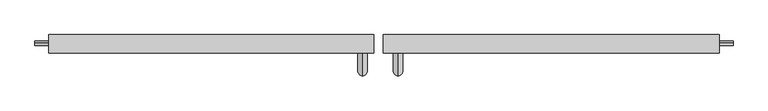
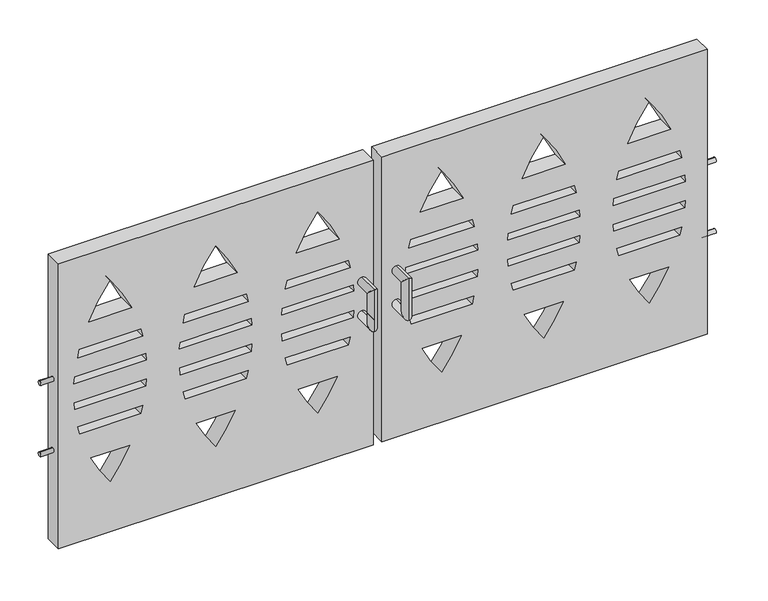
"""IFC4 building model written with IfcOpenShell, lengths in millimetres: proxy geometry."""

from ifc_helpers import new_model, si_unit, point, frame, frame_2d, origin, place, context, project, spatial, polyline, circle_curve, ellipse_curve, trimmed, segment, composite_curve, outline, extrude, source, transform, mapped, element, save
from ifc_brep_helpers import plane_surface, cylinder_surface, advanced_brep


def generic_models_afecbd1f(model_context):
    return source(origin(), model_context, "Body", "SolidModel", [
        extrude(outline(polyline([(0.0, 268.7654616), (1727.2, 268.7654616), (1727.2, -1534.6345384), (0.0, -1534.6345384), (0.0, 268.7654616)]), holes=[composite_curve([segment(trimmed(circle_curve(frame_2d((913.3858921, 735.2120442)), 991.7835907), [point((1315.7032602, -171.3062546))], [point((1522.0610264, -47.8264425))], True, "CARTESIAN"), True, "CONTINUOUS"), segment(trimmed(circle_curve(frame_2d((913.3858921, -830.8649293)), 991.7835907), [point((1522.0610264, -47.8264425))], [point((1315.7032602, 75.6533695))], True, "CARTESIAN"), True, "CONTINUOUS"), segment(polyline([(1315.7032602, 75.6533695), (1315.7032602, -171.3062546)]), True, "CONTINUOUS")], self_intersect=False), composite_curve([segment(trimmed(circle_curve(frame_2d((913.3858921, -830.8649293)), 991.7835907), [point((1167.7706197, 127.7398387))], [point((1120.5108318, 139.0494742))], True, "CARTESIAN"), True, "CONTINUOUS"), segment(polyline([(1120.5108318, 139.0494742), (1120.5108318, -234.7023593)]), True, "CONTINUOUS"), segment(trimmed(circle_curve(frame_2d((913.3858921, 735.2120442)), 991.7835907), [point((1120.5108318, -234.7023593))], [point((1167.7706197, -223.3927238))], True, "CARTESIAN"), True, "CONTINUOUS"), segment(polyline([(1167.7706197, -223.3927238), (1167.7706197, 127.7398387)]), True, "CONTINUOUS")], self_intersect=False), composite_curve([segment(trimmed(circle_curve(frame_2d((913.3858921, -830.8649293)), 991.7835907), [point((1008.9376367, 156.3050434))], [point((969.7809206, 159.3139897))], True, "CARTESIAN"), True, "CONTINUOUS"), segment(polyline([(969.7809206, 159.3139897), (969.7809206, -254.9668748)]), True, "CONTINUOUS"), segment(trimmed(circle_curve(frame_2d((913.3858921, 735.2120442)), 991.7835907), [point((969.7809206, -254.9668748))], [point((1008.9376367, -251.9579284))], True, "CARTESIAN"), True, "CONTINUOUS"), segment(polyline([(1008.9376367, -251.9579284), (1008.9376367, 156.3050434)]), True, "CONTINUOUS")], self_intersect=False), composite_curve([segment(trimmed(circle_curve(frame_2d((913.3858921, -830.8649293)), 991.7835907), [point((853.4628105, 159.1067446))], [point((811.4921317, 155.6706009))], True, "CARTESIAN"), True, "CONTINUOUS"), segment(polyline([(811.4921317, 155.6706009), (811.4921317, -251.323486)]), True, "CONTINUOUS"), segment(trimmed(circle_curve(frame_2d((913.3858921, 735.2120442)), 991.7835907), [point((811.4921317, -251.323486))], [point((853.4628105, -254.7596297))], True, "CARTESIAN"), True, "CONTINUOUS"), segment(polyline([(853.4628105, -254.7596297), (853.4628105, 159.1067446)]), True, "CONTINUOUS")], self_intersect=False), composite_curve([segment(trimmed(circle_curve(frame_2d((913.3858921, -830.8649293)), 991.7835907), [point((700.6764218, 137.8400681))], [point((655.683383, 126.8532483))], True, "CARTESIAN"), True, "CONTINUOUS"), segment(polyline([(655.683383, 126.8532483), (655.683383, -222.5061333)]), True, "CONTINUOUS"), segment(trimmed(circle_curve(frame_2d((913.3858921, 735.2120442)), 991.7835907), [point((655.683383, -222.5061333))], [point((700.6764218, -233.4929532))], True, "CARTESIAN"), True, "CONTINUOUS"), segment(polyline([(700.6764218, -233.4929532), (700.6764218, 137.8400681)]), True, "CONTINUOUS")], self_intersect=False), composite_curve([segment(trimmed(circle_curve(frame_2d((913.3858921, -830.8649293)), 991.7835907), [point((485.5755246, 63.9048625))], [point((304.7107578, -47.8264425))], True, "CARTESIAN"), True, "CONTINUOUS"), segment(trimmed(circle_curve(frame_2d((913.3858921, 735.2120442)), 991.7835907), [point((304.7107578, -47.8264425))], [point((485.5755246, -159.5577476))], True, "CARTESIAN"), True, "CONTINUOUS"), segment(polyline([(485.5755246, -159.5577476), (485.5755246, 63.9048625)]), True, "CONTINUOUS")], self_intersect=False), composite_curve([segment(polyline([(1315.7032602, -510.0774949), (1315.7032602, -757.0371191)]), True, "CONTINUOUS"), segment(trimmed(circle_curve(frame_2d((913.3858921, 149.4811798)), 991.7835907), [point((1315.7032602, -757.0371191))], [point((1522.0610264, -633.557307))], True, "CARTESIAN"), True, "CONTINUOUS"), segment(trimmed(circle_curve(frame_2d((913.3858921, -1416.5957937)), 991.7835907), [point((1522.0610264, -633.557307))], [point((1315.7032602, -510.0774949))], True, "CARTESIAN"), True, "CONTINUOUS")], self_intersect=False), composite_curve([segment(polyline([(1167.7706197, -809.1235882), (1167.7706197, -457.9910257)]), True, "CONTINUOUS"), segment(trimmed(circle_curve(frame_2d((913.3858921, -1416.5957937)), 991.7835907), [point((1167.7706197, -457.9910257))], [point((1120.5108318, -446.6813902))], True, "CARTESIAN"), True, "CONTINUOUS"), segment(polyline([(1120.5108318, -446.6813902), (1120.5108318, -820.4332237)]), True, "CONTINUOUS"), segment(trimmed(circle_curve(frame_2d((913.3858921, 149.4811798)), 991.7835907), [point((1120.5108318, -820.4332237))], [point((1167.7706197, -809.1235882))], True, "CARTESIAN"), True, "CONTINUOUS")], self_intersect=False), composite_curve([segment(polyline([(1008.9376367, -837.6887929), (1008.9376367, -429.4258211)]), True, "CONTINUOUS"), segment(trimmed(circle_curve(frame_2d((913.3858921, -1416.5957937)), 991.7835907), [point((1008.9376367, -429.4258211))], [point((969.7809206, -426.4168748))], True, "CARTESIAN"), True, "CONTINUOUS"), segment(polyline([(969.7809206, -426.4168748), (969.7809206, -840.6977392)]), True, "CONTINUOUS"), segment(trimmed(circle_curve(frame_2d((913.3858921, 149.4811798)), 991.7835907), [point((969.7809206, -840.6977392))], [point((1008.9376367, -837.6887929))], True, "CARTESIAN"), True, "CONTINUOUS")], self_intersect=False), composite_curve([segment(polyline([(853.4628105, -840.4904941), (853.4628105, -426.6241198)]), True, "CONTINUOUS"), segment(trimmed(circle_curve(frame_2d((913.3858921, -1416.5957937)), 991.7835907), [point((853.4628105, -426.6241198))], [point((811.4921317, -430.0602635))], True, "CARTESIAN"), True, "CONTINUOUS"), segment(polyline([(811.4921317, -430.0602635), (811.4921317, -837.0543504)]), True, "CONTINUOUS"), segment(trimmed(circle_curve(frame_2d((913.3858921, 149.4811798)), 991.7835907), [point((811.4921317, -837.0543504))], [point((853.4628105, -840.4904941))], True, "CARTESIAN"), True, "CONTINUOUS")], self_intersect=False), composite_curve([segment(polyline([(700.6764218, -819.2238176), (700.6764218, -447.8907963)]), True, "CONTINUOUS"), segment(trimmed(circle_curve(frame_2d((913.3858921, -1416.5957937)), 991.7835907), [point((700.6764218, -447.8907963))], [point((655.683383, -458.8776162))], True, "CARTESIAN"), True, "CONTINUOUS"), segment(polyline([(655.683383, -458.8776162), (655.683383, -808.2369978)]), True, "CONTINUOUS"), segment(trimmed(circle_curve(frame_2d((913.3858921, 149.4811798)), 991.7835907), [point((655.683383, -808.2369978))], [point((700.6764218, -819.2238176))], True, "CARTESIAN"), True, "CONTINUOUS")], self_intersect=False), composite_curve([segment(polyline([(485.5755246, -745.288612), (485.5755246, -521.8260019)]), True, "CONTINUOUS"), segment(trimmed(circle_curve(frame_2d((913.3858921, -1416.5957937)), 991.7835907), [point((485.5755246, -521.8260019))], [point((304.7107578, -633.557307))], True, "CARTESIAN"), True, "CONTINUOUS"), segment(trimmed(circle_curve(frame_2d((913.3858921, 149.4811798)), 991.7835907), [point((304.7107578, -633.557307))], [point((485.5755246, -745.288612))], True, "CARTESIAN"), True, "CONTINUOUS")], self_intersect=False), composite_curve([segment(trimmed(circle_curve(frame_2d((913.3858921, -455.2996847)), 991.7835907), [point((1315.7032602, -1361.8179835))], [point((1522.0610264, -1238.3381714))], True, "CARTESIAN"), True, "CONTINUOUS"), segment(trimmed(circle_curve(frame_2d((913.3858921, -2021.3766581)), 991.7835907), [point((1522.0610264, -1238.3381714))], [point((1315.7032602, -1114.8583593))], True, "CARTESIAN"), True, "CONTINUOUS"), segment(polyline([(1315.7032602, -1114.8583593), (1315.7032602, -1361.8179835)]), True, "CONTINUOUS")], self_intersect=False), composite_curve([segment(trimmed(circle_curve(frame_2d((913.3858921, -2021.3766581)), 991.7835907), [point((1167.7706197, -1062.7718902))], [point((1120.5108318, -1051.4622546))], True, "CARTESIAN"), True, "CONTINUOUS"), segment(polyline([(1120.5108318, -1051.4622546), (1120.5108318, -1425.2140882)]), True, "CONTINUOUS"), segment(trimmed(circle_curve(frame_2d((913.3858921, -455.2996847)), 991.7835907), [point((1120.5108318, -1425.2140882))], [point((1167.7706197, -1413.9044526))], True, "CARTESIAN"), True, "CONTINUOUS"), segment(polyline([(1167.7706197, -1413.9044526), (1167.7706197, -1062.7718902)]), True, "CONTINUOUS")], self_intersect=False), composite_curve([segment(trimmed(circle_curve(frame_2d((913.3858921, -2021.3766581)), 991.7835907), [point((1008.9376367, -1034.2066855))], [point((969.7809206, -1031.1977392))], True, "CARTESIAN"), True, "CONTINUOUS"), segment(polyline([(969.7809206, -1031.1977392), (969.7809206, -1445.4786036)]), True, "CONTINUOUS"), segment(trimmed(circle_curve(frame_2d((913.3858921, -455.2996847)), 991.7835907), [point((969.7809206, -1445.4786036))], [point((1008.9376367, -1442.4696573))], True, "CARTESIAN"), True, "CONTINUOUS"), segment(polyline([(1008.9376367, -1442.4696573), (1008.9376367, -1034.2066855)]), True, "CONTINUOUS")], self_intersect=False), composite_curve([segment(trimmed(circle_curve(frame_2d((913.3858921, -2021.3766581)), 991.7835907), [point((853.4628105, -1031.4049843))], [point((811.4921317, -1034.8411279))], True, "CARTESIAN"), True, "CONTINUOUS"), segment(polyline([(811.4921317, -1034.8411279), (811.4921317, -1441.8352149)]), True, "CONTINUOUS"), segment(trimmed(circle_curve(frame_2d((913.3858921, -455.2996847)), 991.7835907), [point((811.4921317, -1441.8352149))], [point((853.4628105, -1445.2713585))], True, "CARTESIAN"), True, "CONTINUOUS"), segment(polyline([(853.4628105, -1445.2713585), (853.4628105, -1031.4049843)]), True, "CONTINUOUS")], self_intersect=False), composite_curve([segment(trimmed(circle_curve(frame_2d((913.3858921, -2021.3766581)), 991.7835907), [point((700.6764218, -1052.6716607))], [point((655.683383, -1063.6584806))], True, "CARTESIAN"), True, "CONTINUOUS"), segment(polyline([(655.683383, -1063.6584806), (655.683383, -1413.0178622)]), True, "CONTINUOUS"), segment(trimmed(circle_curve(frame_2d((913.3858921, -455.2996847)), 991.7835907), [point((655.683383, -1413.0178622))], [point((700.6764218, -1424.0046821))], True, "CARTESIAN"), True, "CONTINUOUS"), segment(polyline([(700.6764218, -1424.0046821), (700.6764218, -1052.6716607)]), True, "CONTINUOUS")], self_intersect=False), composite_curve([segment(trimmed(circle_curve(frame_2d((913.3858921, -2021.3766581)), 991.7835907), [point((485.5755246, -1126.6068664))], [point((304.7107578, -1238.3381714))], True, "CARTESIAN"), True, "CONTINUOUS"), segment(trimmed(circle_curve(frame_2d((913.3858921, -455.2996847)), 991.7835907), [point((304.7107578, -1238.3381714))], [point((485.5755246, -1350.0694764))], True, "CARTESIAN"), True, "CONTINUOUS"), segment(polyline([(485.5755246, -1350.0694764), (485.5755246, -1126.6068664)]), True, "CONTINUOUS")], self_intersect=False)]), frame((0.0, -101.6, 0.0), z_axis=(0.0, 1.0, 0.0), x_axis=(0.0, 0.0, 1.0)), (0.0, 0.0, 1.0), 101.6),
        extrude(outline(polyline([(1727.2, 2183.266195), (1727.2, 319.5654616), (0.0, 319.5654616), (0.0, 2183.266195), (1727.2, 2183.266195)]), holes=[composite_curve([segment(polyline([(1315.7032602, 785.0371778), (1315.7032602, 538.0775536)]), True, "CONTINUOUS"), segment(trimmed(circle_curve(frame_2d((913.3858921, 1444.5958525)), 991.7835907), [point((1315.7032602, 538.0775536))], [point((1522.0610264, 661.5573657))], True, "CARTESIAN"), True, "CONTINUOUS"), segment(trimmed(circle_curve(frame_2d((913.3858921, -121.481121)), 991.7835907), [point((1522.0610264, 661.5573657))], [point((1315.7032602, 785.0371778))], True, "CARTESIAN"), True, "CONTINUOUS")], self_intersect=False), composite_curve([segment(polyline([(1167.7706197, 485.9910845), (1167.7706197, 837.1236469)]), True, "CONTINUOUS"), segment(trimmed(circle_curve(frame_2d((913.3858921, -121.481121)), 991.7835907), [point((1167.7706197, 837.1236469))], [point((1120.5108318, 848.4332825))], True, "CARTESIAN"), True, "CONTINUOUS"), segment(polyline([(1120.5108318, 848.4332825), (1120.5108318, 474.681449)]), True, "CONTINUOUS"), segment(trimmed(circle_curve(frame_2d((913.3858921, 1444.5958525)), 991.7835907), [point((1120.5108318, 474.681449))], [point((1167.7706197, 485.9910845))], True, "CARTESIAN"), True, "CONTINUOUS")], self_intersect=False), composite_curve([segment(polyline([(1008.9376367, 457.4258798), (1008.9376367, 865.6888516)]), True, "CONTINUOUS"), segment(trimmed(circle_curve(frame_2d((913.3858921, -121.481121)), 991.7835907), [point((1008.9376367, 865.6888516))], [point((969.7809206, 868.6977979))], True, "CARTESIAN"), True, "CONTINUOUS"), segment(polyline([(969.7809206, 868.6977979), (969.7809206, 454.4169335)]), True, "CONTINUOUS"), segment(trimmed(circle_curve(frame_2d((913.3858921, 1444.5958525)), 991.7835907), [point((969.7809206, 454.4169335))], [point((1008.9376367, 457.4258798))], True, "CARTESIAN"), True, "CONTINUOUS")], self_intersect=False), composite_curve([segment(polyline([(853.4628105, 454.6241786), (853.4628105, 868.4905529)]), True, "CONTINUOUS"), segment(trimmed(circle_curve(frame_2d((913.3858921, -121.481121)), 991.7835907), [point((853.4628105, 868.4905529))], [point((811.4921317, 865.0544092))], True, "CARTESIAN"), True, "CONTINUOUS"), segment(polyline([(811.4921317, 865.0544092), (811.4921317, 458.0603222)]), True, "CONTINUOUS"), segment(trimmed(circle_curve(frame_2d((913.3858921, 1444.5958525)), 991.7835907), [point((811.4921317, 458.0603222))], [point((853.4628105, 454.6241786))], True, "CARTESIAN"), True, "CONTINUOUS")], self_intersect=False), composite_curve([segment(polyline([(700.6764218, 475.890855), (700.6764218, 847.2238764)]), True, "CONTINUOUS"), segment(trimmed(circle_curve(frame_2d((913.3858921, -121.481121)), 991.7835907), [point((700.6764218, 847.2238764))], [point((655.683383, 836.2370565))], True, "CARTESIAN"), True, "CONTINUOUS"), segment(polyline([(655.683383, 836.2370565), (655.683383, 486.8776749)]), True, "CONTINUOUS"), segment(trimmed(circle_curve(frame_2d((913.3858921, 1444.5958525)), 991.7835907), [point((655.683383, 486.8776749))], [point((700.6764218, 475.890855))], True, "CARTESIAN"), True, "CONTINUOUS")], self_intersect=False), composite_curve([segment(polyline([(485.5755246, 549.8260607), (485.5755246, 773.2886707)]), True, "CONTINUOUS"), segment(trimmed(circle_curve(frame_2d((913.3858921, -121.481121)), 991.7835907), [point((485.5755246, 773.2886707))], [point((304.7107578, 661.5573657))], True, "CARTESIAN"), True, "CONTINUOUS"), segment(trimmed(circle_curve(frame_2d((913.3858921, 1444.5958525)), 991.7835907), [point((304.7107578, 661.5573657))], [point((485.5755246, 549.8260607))], True, "CARTESIAN"), True, "CONTINUOUS")], self_intersect=False), composite_curve([segment(trimmed(circle_curve(frame_2d((913.3858921, 2030.3267169)), 991.7835907), [point((1315.7032602, 1123.8084181))], [point((1522.0610264, 1247.2882301))], True, "CARTESIAN"), True, "CONTINUOUS"), segment(trimmed(circle_curve(frame_2d((913.3858921, 464.2497434)), 991.7835907), [point((1522.0610264, 1247.2882301))], [point((1315.7032602, 1370.7680422))], True, "CARTESIAN"), True, "CONTINUOUS"), segment(polyline([(1315.7032602, 1370.7680422), (1315.7032602, 1123.8084181)]), True, "CONTINUOUS")], self_intersect=False), composite_curve([segment(trimmed(circle_curve(frame_2d((913.3858921, 464.2497434)), 991.7835907), [point((1167.7706197, 1422.8545114))], [point((1120.5108318, 1434.1641469))], True, "CARTESIAN"), True, "CONTINUOUS"), segment(polyline([(1120.5108318, 1434.1641469), (1120.5108318, 1060.4123134)]), True, "CONTINUOUS"), segment(trimmed(circle_curve(frame_2d((913.3858921, 2030.3267169)), 991.7835907), [point((1120.5108318, 1060.4123134))], [point((1167.7706197, 1071.7219489))], True, "CARTESIAN"), True, "CONTINUOUS"), segment(polyline([(1167.7706197, 1071.7219489), (1167.7706197, 1422.8545114)]), True, "CONTINUOUS")], self_intersect=False), composite_curve([segment(trimmed(circle_curve(frame_2d((913.3858921, 464.2497434)), 991.7835907), [point((1008.9376367, 1451.419716))], [point((969.7809206, 1454.4286624))], True, "CARTESIAN"), True, "CONTINUOUS"), segment(polyline([(969.7809206, 1454.4286624), (969.7809206, 1040.1477979)]), True, "CONTINUOUS"), segment(trimmed(circle_curve(frame_2d((913.3858921, 2030.3267169)), 991.7835907), [point((969.7809206, 1040.1477979))], [point((1008.9376367, 1043.1567442))], True, "CARTESIAN"), True, "CONTINUOUS"), segment(polyline([(1008.9376367, 1043.1567442), (1008.9376367, 1451.419716)]), True, "CONTINUOUS")], self_intersect=False), composite_curve([segment(trimmed(circle_curve(frame_2d((913.3858921, 464.2497434)), 991.7835907), [point((853.4628105, 1454.2214173))], [point((811.4921317, 1450.7852736))], True, "CARTESIAN"), True, "CONTINUOUS"), segment(polyline([(811.4921317, 1450.7852736), (811.4921317, 1043.7911867)]), True, "CONTINUOUS"), segment(trimmed(circle_curve(frame_2d((913.3858921, 2030.3267169)), 991.7835907), [point((811.4921317, 1043.7911867))], [point((853.4628105, 1040.355043))], True, "CARTESIAN"), True, "CONTINUOUS"), segment(polyline([(853.4628105, 1040.355043), (853.4628105, 1454.2214173)]), True, "CONTINUOUS")], self_intersect=False), composite_curve([segment(trimmed(circle_curve(frame_2d((913.3858921, 464.2497434)), 991.7835907), [point((700.6764218, 1432.9547408))], [point((655.683383, 1421.9679209))], True, "CARTESIAN"), True, "CONTINUOUS"), segment(polyline([(655.683383, 1421.9679209), (655.683383, 1072.6085394)]), True, "CONTINUOUS"), segment(trimmed(circle_curve(frame_2d((913.3858921, 2030.3267169)), 991.7835907), [point((655.683383, 1072.6085394))], [point((700.6764218, 1061.6217195))], True, "CARTESIAN"), True, "CONTINUOUS"), segment(polyline([(700.6764218, 1061.6217195), (700.6764218, 1432.9547408)]), True, "CONTINUOUS")], self_intersect=False), composite_curve([segment(trimmed(circle_curve(frame_2d((913.3858921, 464.2497434)), 991.7835907), [point((485.5755246, 1359.0195352))], [point((304.7107578, 1247.2882301))], True, "CARTESIAN"), True, "CONTINUOUS"), segment(trimmed(circle_curve(frame_2d((913.3858921, 2030.3267169)), 991.7835907), [point((304.7107578, 1247.2882301))], [point((485.5755246, 1135.5569251))], True, "CARTESIAN"), True, "CONTINUOUS"), segment(polyline([(485.5755246, 1135.5569251), (485.5755246, 1359.0195352)]), True, "CONTINUOUS")], self_intersect=False), composite_curve([segment(polyline([(1315.7032602, 1975.5489067), (1315.7032602, 1728.5892825)]), True, "CONTINUOUS"), segment(trimmed(circle_curve(frame_2d((913.3858921, 2635.1075813)), 991.7835907), [point((1315.7032602, 1728.5892825))], [point((1522.0610264, 1852.0690946))], True, "CARTESIAN"), True, "CONTINUOUS"), segment(trimmed(circle_curve(frame_2d((913.3858921, 1069.0306078)), 991.7835907), [point((1522.0610264, 1852.0690946))], [point((1315.7032602, 1975.5489067))], True, "CARTESIAN"), True, "CONTINUOUS")], self_intersect=False), composite_curve([segment(polyline([(1167.7706197, 1676.5028134), (1167.7706197, 2027.6353758)]), True, "CONTINUOUS"), segment(trimmed(circle_curve(frame_2d((913.3858921, 1069.0306078)), 991.7835907), [point((1167.7706197, 2027.6353758))], [point((1120.5108318, 2038.9450113))], True, "CARTESIAN"), True, "CONTINUOUS"), segment(polyline([(1120.5108318, 2038.9450113), (1120.5108318, 1665.1931778)]), True, "CONTINUOUS"), segment(trimmed(circle_curve(frame_2d((913.3858921, 2635.1075813)), 991.7835907), [point((1120.5108318, 1665.1931778))], [point((1167.7706197, 1676.5028134))], True, "CARTESIAN"), True, "CONTINUOUS")], self_intersect=False), composite_curve([segment(polyline([(1008.9376367, 1647.9376087), (1008.9376367, 2056.2005805)]), True, "CONTINUOUS"), segment(trimmed(circle_curve(frame_2d((913.3858921, 1069.0306078)), 991.7835907), [point((1008.9376367, 2056.2005805))], [point((969.7809206, 2059.2095268))], True, "CARTESIAN"), True, "CONTINUOUS"), segment(polyline([(969.7809206, 2059.2095268), (969.7809206, 1644.9286624)]), True, "CONTINUOUS"), segment(trimmed(circle_curve(frame_2d((913.3858921, 2635.1075813)), 991.7835907), [point((969.7809206, 1644.9286624))], [point((1008.9376367, 1647.9376087))], True, "CARTESIAN"), True, "CONTINUOUS")], self_intersect=False), composite_curve([segment(polyline([(853.4628105, 1645.1359074), (853.4628105, 2059.0022817)]), True, "CONTINUOUS"), segment(trimmed(circle_curve(frame_2d((913.3858921, 1069.0306078)), 991.7835907), [point((853.4628105, 2059.0022817))], [point((811.4921317, 2055.566138))], True, "CARTESIAN"), True, "CONTINUOUS"), segment(polyline([(811.4921317, 2055.566138), (811.4921317, 1648.5720511)]), True, "CONTINUOUS"), segment(trimmed(circle_curve(frame_2d((913.3858921, 2635.1075813)), 991.7835907), [point((811.4921317, 1648.5720511))], [point((853.4628105, 1645.1359074))], True, "CARTESIAN"), True, "CONTINUOUS")], self_intersect=False), composite_curve([segment(polyline([(700.6764218, 1666.4025839), (700.6764218, 2037.7356052)]), True, "CONTINUOUS"), segment(trimmed(circle_curve(frame_2d((913.3858921, 1069.0306078)), 991.7835907), [point((700.6764218, 2037.7356052))], [point((655.683383, 2026.7487854))], True, "CARTESIAN"), True, "CONTINUOUS"), segment(polyline([(655.683383, 2026.7487854), (655.683383, 1677.3894038)]), True, "CONTINUOUS"), segment(trimmed(circle_curve(frame_2d((913.3858921, 2635.1075813)), 991.7835907), [point((655.683383, 1677.3894038))], [point((700.6764218, 1666.4025839))], True, "CARTESIAN"), True, "CONTINUOUS")], self_intersect=False), composite_curve([segment(polyline([(485.5755246, 1740.3377895), (485.5755246, 1963.8003996)]), True, "CONTINUOUS"), segment(trimmed(circle_curve(frame_2d((913.3858921, 1069.0306078)), 991.7835907), [point((485.5755246, 1963.8003996))], [point((304.7107578, 1852.0690946))], True, "CARTESIAN"), True, "CONTINUOUS"), segment(trimmed(circle_curve(frame_2d((913.3858921, 2635.1075813)), 991.7835907), [point((304.7107578, 1852.0690946))], [point((485.5755246, 1740.3377895))], True, "CARTESIAN"), True, "CONTINUOUS")], self_intersect=False)]), frame((0.0, -101.6, 0.0), z_axis=(0.0, 1.0, 0.0), x_axis=(0.0, 0.0, 1.0)), (0.0, 0.0, 1.0), 101.6),
        advanced_brep(
        [(205.2654616, -101.6, 1039.4610264), (205.2654616, -101.6, 988.6610264), (205.2654616, -101.6, 785.4610264), (205.2654616, -101.6, 836.2610264), (205.2654616, -228.6, 1039.4610264), (205.2654616, -177.8, 988.6610264), (205.2654616, -228.6, 785.4610264), (205.2654616, -177.8, 836.2610264)],
        [
            (0, 1, circle_curve(frame((205.2654616, -101.6, 1014.0610264), z_axis=(0.0, 1.0, 0.0), x_axis=(0.0, 0.0, -1.0)), 25.4)),
            (1, 0, circle_curve(frame((205.2654616, -101.6, 1014.0610264), z_axis=(0.0, 1.0, 0.0), x_axis=(0.0, 0.0, -1.0)), 25.4)),
            (2, 3, circle_curve(frame((205.2654616, -101.6, 810.8610264), z_axis=(0.0, 1.0, 0.0), x_axis=(0.0, 0.0, 1.0)), 25.4)),
            (3, 2, circle_curve(frame((205.2654616, -101.6, 810.8610264), z_axis=(0.0, 1.0, 0.0), x_axis=(0.0, 0.0, 1.0)), 25.4)),
            (0, 4),
            (4, 5, ellipse_curve(frame((205.2654616, -203.2, 1014.0610264), z_axis=(0.0, 0.7071067811865495, 0.7071067811865455), x_axis=(0.0, 0.7071067811865457, -0.7071067811865493)), 35.9210245, 25.4)),
            (5, 1),
            (5, 4, ellipse_curve(frame((205.2654616, -203.2, 1014.0610264), z_axis=(0.0, 0.7071067811865495, 0.7071067811865455), x_axis=(0.0, 0.7071067811865457, -0.7071067811865493)), 35.9210245, 25.4)),
            (4, 6),
            (6, 7, ellipse_curve(frame((205.2654616, -203.2, 810.8610264), z_axis=(0.0, -0.7071067811865457, 0.7071067811865495), x_axis=(0.0, 0.7071067811865496, 0.7071067811865455)), 35.9210245, 25.4)),
            (7, 5),
            (7, 6, ellipse_curve(frame((205.2654616, -203.2, 810.8610264), z_axis=(0.0, -0.7071067811865457, 0.7071067811865495), x_axis=(0.0, 0.7071067811865496, 0.7071067811865455)), 35.9210245, 25.4)),
            (6, 2),
            (3, 7),
        ],
        [
            plane_surface(frame((205.2654616, -101.6, 1014.0610264), z_axis=(0.0, 1.0, 0.0), x_axis=(1.0, 0.0, 0.0))),
            plane_surface(frame((205.2654616, -101.6, 810.8610264), z_axis=(0.0, 1.0, 0.0), x_axis=(1.0, 0.0, 0.0))),
            cylinder_surface(frame((205.2654616, -101.6, 1014.0610264), z_axis=(0.0, 1.0, 0.0), x_axis=(0.0, 0.0, -1.0)), 25.4),
            cylinder_surface(frame((205.2654616, -203.2, 1014.0610264), z_axis=(0.0, 0.0, 1.0), x_axis=(0.0, 1.0, 0.0)), 25.4),
            cylinder_surface(frame((205.2654616, -203.2, 810.8610264), z_axis=(0.0, -1.0, 0.0), x_axis=(0.0, 0.0, 1.0)), 25.4),
        ],
        [
            (0, [[1, 2]]),
            (1, [[3, 4]]),
            (2, [[-1, 5, 6, 7]]),
            (2, [[-2, -7, 8, -5]]),
            (3, [[-6, 9, 10, 11]]),
            (3, [[-8, -11, 12, -9]]),
            (4, [[-10, 13, -4, 14]]),
            (4, [[-12, -14, -3, -13]]),
        ],
    ),
        advanced_brep(
        [(402.1154616, -101.6, 1039.4610264), (402.1154616, -101.6, 988.6610264), (402.1154616, -101.6, 785.4610264), (402.1154616, -101.6, 836.2610264), (402.1154616, -228.6, 1039.4610264), (402.1154616, -177.8, 988.6610264), (402.1154616, -228.6, 785.4610264), (402.1154616, -177.8, 836.2610264)],
        [
            (0, 1, circle_curve(frame((402.1154616, -101.6, 1014.0610264), z_axis=(0.0, 1.0, 0.0), x_axis=(0.0, 0.0, -1.0)), 25.4)),
            (1, 0, circle_curve(frame((402.1154616, -101.6, 1014.0610264), z_axis=(0.0, 1.0, 0.0), x_axis=(0.0, 0.0, -1.0)), 25.4)),
            (2, 3, circle_curve(frame((402.1154616, -101.6, 810.8610264), z_axis=(0.0, 1.0, 0.0), x_axis=(0.0, 0.0, 1.0)), 25.4)),
            (3, 2, circle_curve(frame((402.1154616, -101.6, 810.8610264), z_axis=(0.0, 1.0, 0.0), x_axis=(0.0, 0.0, 1.0)), 25.4)),
            (0, 4),
            (4, 5, ellipse_curve(frame((402.1154616, -203.2, 1014.0610264), z_axis=(0.0, 0.7071067811865495, 0.7071067811865455), x_axis=(0.0, 0.7071067811865457, -0.7071067811865493)), 35.9210245, 25.4)),
            (5, 1),
            (5, 4, ellipse_curve(frame((402.1154616, -203.2, 1014.0610264), z_axis=(0.0, 0.7071067811865495, 0.7071067811865455), x_axis=(0.0, 0.7071067811865457, -0.7071067811865493)), 35.9210245, 25.4)),
            (4, 6),
            (6, 7, ellipse_curve(frame((402.1154616, -203.2, 810.8610264), z_axis=(0.0, -0.7071067811865457, 0.7071067811865495), x_axis=(0.0, 0.7071067811865496, 0.7071067811865455)), 35.9210245, 25.4)),
            (7, 5),
            (7, 6, ellipse_curve(frame((402.1154616, -203.2, 810.8610264), z_axis=(0.0, -0.7071067811865457, 0.7071067811865495), x_axis=(0.0, 0.7071067811865496, 0.7071067811865455)), 35.9210245, 25.4)),
            (6, 2),
            (3, 7),
        ],
        [
            plane_surface(frame((402.1154616, -101.6, 1014.0610264), z_axis=(0.0, 1.0, 0.0), x_axis=(1.0, 0.0, 0.0))),
            plane_surface(frame((402.1154616, -101.6, 810.8610264), z_axis=(0.0, 1.0, 0.0), x_axis=(1.0, 0.0, 0.0))),
            cylinder_surface(frame((402.1154616, -101.6, 1014.0610264), z_axis=(0.0, 1.0, 0.0), x_axis=(0.0, 0.0, -1.0)), 25.4),
            cylinder_surface(frame((402.1154616, -203.2, 1014.0610264), z_axis=(0.0, 0.0, 1.0), x_axis=(0.0, 1.0, 0.0)), 25.4),
            cylinder_surface(frame((402.1154616, -203.2, 810.8610264), z_axis=(0.0, -1.0, 0.0), x_axis=(0.0, 0.0, 1.0)), 25.4),
        ],
        [
            (0, [[1, 2]]),
            (1, [[3, 4]]),
            (2, [[-1, 5, 6, 7]]),
            (2, [[-2, -7, 8, -5]]),
            (3, [[-6, 9, 10, 11]]),
            (3, [[-8, -11, 12, -9]]),
            (4, [[-10, 13, -4, 14]]),
            (4, [[-12, -14, -3, -13]]),
        ],
    ),
        extrude(outline(composite_curve([segment(trimmed(circle_curve(frame_2d((-47.1865605, 998.9501685)), 12.7), [point((-47.1865605, 1011.6501685))], [point((-47.1865605, 986.2501685))], False, "CARTESIAN"), True, "CONTINUOUS"), segment(trimmed(circle_curve(frame_2d((-47.1865605, 998.9501685)), 12.7), [point((-47.1865605, 986.2501685))], [point((-47.1865605, 1011.6501685))], False, "CARTESIAN"), True, "CONTINUOUS")], self_intersect=False)), frame((2183.266195, 0.0, 0.0), z_axis=(1.0, 0.0, 0.0), x_axis=(0.0, 1.0, 0.0)), (0.0, 0.0, 1.0), 76.2),
        extrude(outline(composite_curve([segment(trimmed(circle_curve(frame_2d((-47.1865605, 567.1501685)), 12.7), [point((-47.1865605, 579.8501685))], [point((-47.1865605, 554.4501685))], False, "CARTESIAN"), True, "CONTINUOUS"), segment(trimmed(circle_curve(frame_2d((-47.1865605, 567.1501685)), 12.7), [point((-47.1865605, 554.4501685))], [point((-47.1865605, 579.8501685))], False, "CARTESIAN"), True, "CONTINUOUS")], self_intersect=False)), frame((2183.266195, 0.0, 0.0), z_axis=(1.0, 0.0, 0.0), x_axis=(0.0, 1.0, 0.0)), (0.0, 0.0, 1.0), 76.2),
        extrude(outline(composite_curve([segment(trimmed(circle_curve(frame_2d((-47.1865605, 998.9501685)), 12.7), [point((-47.1865605, 1011.6501685))], [point((-47.1865605, 986.2501685))], False, "CARTESIAN"), True, "CONTINUOUS"), segment(trimmed(circle_curve(frame_2d((-47.1865605, 998.9501685)), 12.7), [point((-47.1865605, 986.2501685))], [point((-47.1865605, 1011.6501685))], False, "CARTESIAN"), True, "CONTINUOUS")], self_intersect=False)), frame((-1610.8345384, 0.0, 0.0), z_axis=(1.0, 0.0, 0.0), x_axis=(0.0, 1.0, 0.0)), (0.0, 0.0, 1.0), 76.2),
        extrude(outline(composite_curve([segment(trimmed(circle_curve(frame_2d((-47.1865605, 567.1501685)), 12.7), [point((-47.1865605, 579.8501685))], [point((-47.1865605, 554.4501685))], False, "CARTESIAN"), True, "CONTINUOUS"), segment(trimmed(circle_curve(frame_2d((-47.1865605, 567.1501685)), 12.7), [point((-47.1865605, 554.4501685))], [point((-47.1865605, 579.8501685))], False, "CARTESIAN"), True, "CONTINUOUS")], self_intersect=False)), frame((-1610.8345384, 0.0, 0.0), z_axis=(1.0, 0.0, 0.0), x_axis=(0.0, 1.0, 0.0)), (0.0, 0.0, 1.0), 76.2),
    ])


if __name__ == "__main__":
    model = new_model("IFC4")
    model_context = context("Model", 3, world=origin())
    ifc_project = project(units=[si_unit("LENGTHUNIT", "METRE", prefix="MILLI")], contexts=[model_context])
    site = spatial("IfcSite", under=ifc_project)
    building = spatial("IfcBuilding", under=site)
    placement = place(None, origin())
    generic_models_shape = generic_models_afecbd1f(model_context)
    element("IfcBuildingElementProxy", 1, Name="Generic Models", at=placement, inside=building, context=model_context, shape_type="MappedRepresentation", body=[
        mapped(generic_models_shape, transform((0.0, 0.0, 0.0), x_axis=(1.0, 0.0, 0.0), y_axis=(0.0, 1.0, 0.0), z_axis=(0.0, 0.0, 1.0))),
    ])
    save(model, "model.ifc")

# Revit data of these elements
# Type
#   Default Elevation = 0
# Element 1 (IfcBuildingElementProxy)
#   Materials on its faces: "GATE"
# Materials
#   "GATE": class "Generic", colour RGB 120 120 120, transparency 0, Cost = 0
